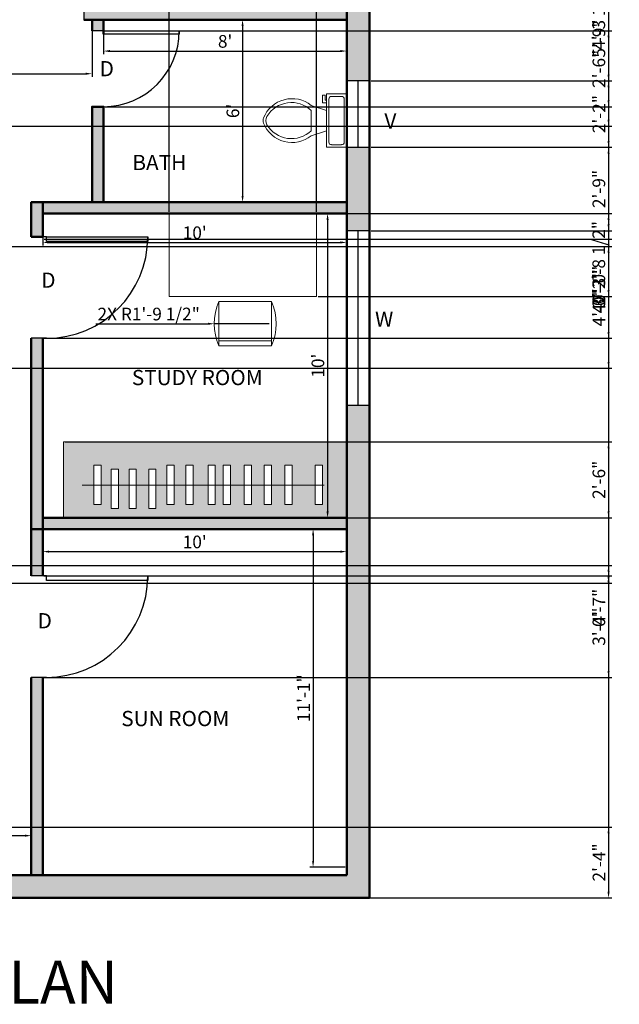
# Model space of a CAD drawing. Units: inches. Extents: x 2064 to 2999, y 1440 to 2089.
# Tile 6 of 7: x 2763 to 2999, y 1446 to 1835. Entities that reach past the tile are written whole.
import ezdxf

# ---------------------------------------------------------------- set-up
doc = ezdxf.new("R2010")
doc.units = ezdxf.units.IN
for name, color, linetype, lineweight in [('A-ANNO-DIMS', 2, 'Continuous', 18), ('A-ANNO-TEXT', 3, 'Continuous', 18), ('A-AREA-IDEN', 7, 'Continuous', 18), ('A-DOOR', 4, 'Continuous', 25), ('A-FLOR-FIXT', 9, 'Continuous', 18), ('A-FURN', 8, 'Continuous', 18), ('A-FURN-PATT', 252, 'Continuous', 13), ('A-GLAZ', 3, 'Continuous', 25), ('A-WALL', 7, 'Continuous', 50), ('A-WALL-PATT', 8, 'Continuous', 13)]:
    doc.layers.add(name, color=color, linetype=linetype, lineweight=lineweight)
doc.styles.get("Standard").update_dxf_attribs({"font": 'arial.ttf'})
doc.dimstyles.new('ISO-25', dxfattribs={"dimtxt": 5, "dimasz": 2.5, "dimexe": 1.25, "dimexo": 0.625, "dimtad": 1, "dimdec": 0, "dimlunit": 4, "dimtxsty": 'Standard', "dimcen": 2.5, "dimadec": 0, "dimazin": 0, "dimtfac": 1, "dimtdec": 0, "dimtmove": 0, "dimatfit": 3, "dimfxl": 1, "dimarcsym": 0})

# ---------------------------------------------------------------- blocks, each defined once
blk = doc.blocks.new('*U2')
for p, q in [((0, 0), (0, -6)), ((40, 0), (40, -6))]:
    blk.add_line(p, q)
blk.add_lwpolyline([(0, 0), (0, 40), (1.75, 40), (1.75, 0)], close=True)
blk.add_arc((0, 0), 40, 0, 90)
blk = doc.blocks.new('*U4')
for p, q in [((9.5, -6), (9.5, -2)), ((-10, -8.5), (-8, -8.5)), ((-10, -9.5), (-10, -8.5)), ((-7, -9.5), (-10, -9.5)), ((-8, -8.5), (-8, -8)), ((-7, -8), (-7, -9.5)), ((-4, -8), (-6, -14)), ((4, -8), (6, -14)), ((4, -14), (-4, -14))]:
    blk.add_line(p, q)
blk.add_lwpolyline([(10.5, -8), (10.5, 0), (-10.5, 0), (-10.5, -8)], close=True)
for points in [[(-9.5, -2), (-9.5, -6)], [(8.5, -1), (-8.5, -1)], [(-8.5, -7), (8.5, -7)]]:
    blk.add_lwpolyline(points)
for centre, radius, start, end in [((-8.62, -1.88), 0.884, 81.8699, 188.1301), ((8.62, -1.88), 0.884, 351.8699, 98.1301), ((-8.62, -6.12), 0.884, 171.8699, 278.1301), ((8.62, -6.12), 0.884, 261.8699, 8.1301), ((3.52, -21.58), 12.17, 141.4691, 247.9714), ((4.2, -21.82), 11.33, 136.3677, 238.9468), ((-3.52, -21.58), 12.17, 292.0284, 38.5307), ((-4.2, -21.82), 11.33, 301.053, 43.6321), ((0, -27.88), 4, 245.7318, 294.2682), ((0, -29), 4, 254.8605, 285.1395)]:
    blk.add_arc(centre, radius, start, end)
blk = doc.blocks.new('*D25')
at = {"layer": 'A-ANNO-DIMS', "color": 0, "lineweight": -2, "transparency": 16777216}
for p, q in [((2891.25, 1834.57), (2849.51, 1834.57)), ((2850.76, 1832.07), (2850.76, 1765.07)), ((2891.25, 1762.57), (2849.51, 1762.57))]:
    blk.add_line(p, q, dxfattribs=at)
at = {"layer": 'A-ANNO-DIMS', "color": 0, "transparency": 16777216}
for points in [[(2850.35, 1832.07), (2851.18, 1832.07), (2850.76, 1834.57)], [(2850.35, 1765.07), (2851.18, 1765.07), (2850.76, 1762.57)]]:
    blk.add_solid(points, dxfattribs=at)
at = {"layer": 'Defpoints', "color": 0, "transparency": 16777216}
for p in [(2891.87, 1834.57), (2850.76, 1762.57), (2891.87, 1762.57)]:
    blk.add_point(p, dxfattribs=at)
at = {"layer": 'A-ANNO-DIMS', "color": 0, "transparency": 16777216, "insert": (2847.58, 1798.57), "char_height": 5, "attachment_point": 5, "rotation": 90}
blk.add_mtext("6'", dxfattribs=at)
blk = doc.blocks.new('*D26')
at = {"layer": 'A-ANNO-DIMS', "color": 0, "lineweight": -2, "transparency": 16777216}
for p, q in [((2795.87, 1833.95), (2795.87, 1820.94)), ((2891.87, 1833.95), (2891.87, 1820.94)), ((2798.37, 1822.19), (2889.37, 1822.19))]:
    blk.add_line(p, q, dxfattribs=at)
at = {"layer": 'A-ANNO-DIMS', "color": 0, "transparency": 16777216}
for points in [[(2798.37, 1822.61), (2798.37, 1821.78), (2795.87, 1822.19)], [(2889.37, 1822.61), (2889.37, 1821.78), (2891.87, 1822.19)]]:
    blk.add_solid(points, dxfattribs=at)
at = {"layer": 'Defpoints', "color": 0, "transparency": 16777216}
for p in [(2795.87, 1834.57), (2891.87, 1834.57), (2891.87, 1822.19)]:
    blk.add_point(p, dxfattribs=at)
at = {"layer": 'A-ANNO-DIMS', "color": 0, "transparency": 16777216, "insert": (2843.87, 1825.37), "char_height": 5, "attachment_point": 5}
blk.add_mtext("8'", dxfattribs=at)
blk = doc.blocks.new('*D27')
at = {"layer": 'A-ANNO-DIMS', "color": 0, "lineweight": -2, "transparency": 16777216}
for p, q in [((2771.87, 1757.45), (2771.87, 1745.43)), ((2891.87, 1757.45), (2891.87, 1745.43)), ((2774.37, 1746.68), (2889.37, 1746.68))]:
    blk.add_line(p, q, dxfattribs=at)
at = {"layer": 'A-ANNO-DIMS', "color": 0, "transparency": 16777216}
for points in [[(2774.37, 1747.1), (2774.37, 1746.27), (2771.87, 1746.68)], [(2889.37, 1747.1), (2889.37, 1746.27), (2891.87, 1746.68)]]:
    blk.add_solid(points, dxfattribs=at)
at = {"layer": 'Defpoints', "color": 0, "transparency": 16777216}
for p in [(2771.87, 1758.07), (2891.87, 1758.07), (2891.87, 1746.68)]:
    blk.add_point(p, dxfattribs=at)
at = {"layer": 'A-ANNO-DIMS', "color": 0, "transparency": 16777216, "insert": (2831.87, 1749.86), "char_height": 5, "attachment_point": 5}
blk.add_mtext("10'", dxfattribs=at)
blk = doc.blocks.new('*D28')
at = {"layer": 'A-ANNO-DIMS', "color": 0, "lineweight": -2, "transparency": 16777216}
for p, q in [((2891.25, 1758.07), (2883.07, 1758.07)), ((2884.32, 1755.57), (2884.32, 1640.57)), ((2891.25, 1638.07), (2883.07, 1638.07))]:
    blk.add_line(p, q, dxfattribs=at)
at = {"layer": 'A-ANNO-DIMS', "color": 0, "transparency": 16777216}
for points in [[(2883.9, 1755.57), (2884.73, 1755.57), (2884.32, 1758.07)], [(2883.9, 1640.57), (2884.73, 1640.57), (2884.32, 1638.07)]]:
    blk.add_solid(points, dxfattribs=at)
at = {"layer": 'Defpoints', "color": 0, "transparency": 16777216}
for p in [(2891.87, 1758.07), (2884.32, 1638.07), (2891.87, 1638.07)]:
    blk.add_point(p, dxfattribs=at)
at = {"layer": 'A-ANNO-DIMS', "color": 0, "transparency": 16777216, "insert": (2881.14, 1698.07), "char_height": 5, "attachment_point": 5, "rotation": 90}
blk.add_mtext("10'", dxfattribs=at)
blk = doc.blocks.new('*D29')
at = {"layer": 'A-ANNO-DIMS', "color": 0, "lineweight": -2, "transparency": 16777216}
for p, q in [((2771.87, 1632.95), (2771.87, 1623.44)), ((2891.87, 1632.95), (2891.87, 1623.44)), ((2774.37, 1624.69), (2889.37, 1624.69))]:
    blk.add_line(p, q, dxfattribs=at)
at = {"layer": 'A-ANNO-DIMS', "color": 0, "transparency": 16777216}
for points in [[(2774.37, 1625.1), (2774.37, 1624.27), (2771.87, 1624.69)], [(2889.37, 1625.1), (2889.37, 1624.27), (2891.87, 1624.69)]]:
    blk.add_solid(points, dxfattribs=at)
at = {"layer": 'Defpoints', "color": 0, "transparency": 16777216}
for p in [(2771.87, 1633.57), (2891.87, 1633.57), (2891.87, 1624.69)]:
    blk.add_point(p, dxfattribs=at)
at = {"layer": 'A-ANNO-DIMS', "color": 0, "transparency": 16777216, "insert": (2831.87, 1627.86), "char_height": 5, "attachment_point": 5}
blk.add_mtext("10'", dxfattribs=at)
blk = doc.blocks.new('*D30')
at = {"layer": 'A-ANNO-DIMS', "color": 0, "lineweight": -2, "transparency": 16777216}
for p, q in [((2891.25, 1633.57), (2877.35, 1633.57)), ((2878.6, 1631.07), (2878.6, 1502.68)), ((2891.25, 1500.18), (2877.35, 1500.18))]:
    blk.add_line(p, q, dxfattribs=at)
at = {"layer": 'A-ANNO-DIMS', "color": 0, "transparency": 16777216}
for points in [[(2878.19, 1631.07), (2879.02, 1631.07), (2878.6, 1633.57)], [(2878.19, 1502.68), (2879.02, 1502.68), (2878.6, 1500.18)]]:
    blk.add_solid(points, dxfattribs=at)
at = {"layer": 'Defpoints', "color": 0, "transparency": 16777216}
for p in [(2891.87, 1633.57), (2878.6, 1500.18), (2891.87, 1500.18)]:
    blk.add_point(p, dxfattribs=at)
at = {"layer": 'A-ANNO-DIMS', "color": 0, "transparency": 16777216, "insert": (2875.47, 1566.88), "char_height": 5, "attachment_point": 5, "rotation": 90}
blk.add_mtext('11\'-1"', dxfattribs=at)
blk = doc.blocks.new('*D31')
at = {"layer": 'A-ANNO-DIMS', "color": 0, "lineweight": -2, "transparency": 16777216}
for p, q in [((2549.87, 1497.7), (2549.87, 1513.87)), ((2552.37, 1512.62), (2764.87, 1512.62)), ((2767.37, 1497.7), (2767.37, 1513.87))]:
    blk.add_line(p, q, dxfattribs=at)
at = {"layer": 'A-ANNO-DIMS', "color": 0, "transparency": 16777216}
for points in [[(2552.37, 1513.04), (2552.37, 1512.2), (2549.87, 1512.62)], [(2764.87, 1513.04), (2764.87, 1512.2), (2767.37, 1512.62)]]:
    blk.add_solid(points, dxfattribs=at)
at = {"layer": 'Defpoints', "color": 0, "transparency": 16777216}
for p in [(2767.37, 1512.62), (2549.87, 1497.07), (2767.37, 1497.07)]:
    blk.add_point(p, dxfattribs=at)
at = {"layer": 'A-ANNO-DIMS', "color": 0, "transparency": 16777216, "insert": (2658.62, 1515.8), "char_height": 5, "attachment_point": 5}
blk.add_mtext('18\'-2"', dxfattribs=at)
blk = doc.blocks.new('*D33')
at = {"layer": 'A-ANNO-DIMS', "color": 0, "lineweight": -2, "transparency": 16777216}
for p, q in [((2616.69, 1833.95), (2616.69, 1812)), ((2791.37, 1833.95), (2791.37, 1812)), ((2619.19, 1813.25), (2788.87, 1813.25))]:
    blk.add_line(p, q, dxfattribs=at)
at = {"layer": 'A-ANNO-DIMS', "color": 0, "transparency": 16777216}
for points in [[(2619.19, 1813.67), (2619.19, 1812.84), (2616.69, 1813.25)], [(2788.87, 1813.67), (2788.87, 1812.84), (2791.37, 1813.25)]]:
    blk.add_solid(points, dxfattribs=at)
at = {"layer": 'Defpoints', "color": 0, "transparency": 16777216}
for p in [(2616.69, 1834.57), (2791.37, 1834.57), (2791.37, 1813.25)]:
    blk.add_point(p, dxfattribs=at)
at = {"layer": 'A-ANNO-DIMS', "color": 0, "transparency": 16777216, "insert": (2704.03, 1816.39), "char_height": 5, "attachment_point": 5}
blk.add_mtext('14\'-7"', dxfattribs=at)
blk = doc.blocks.new('BOOK')
for p, q in [((0, 3.13), (0, 15.5)), ((0, 15.5), (0, 0)), ((2.86, 15.5), (0, 15.5)), ((2.86, 0), (2.86, 15.5)), ((0, 0), (2.86, 0))]:
    blk.add_line(p, q)
blk = doc.blocks.new('WIN-69')
blk.add_line((4.5, 0), (4.5, 68.8))
blk.add_lwpolyline([(0, 0), (9, 0), (9, 68.8), (0, 68.8)], close=True)
blk = doc.blocks.new('*D83')
at = {"layer": 'A-ANNO-DIMS', "color": 0, "lineweight": -2, "transparency": 16777216}
for p, q in [((2901.5, 1968.07), (2996.47, 1968.07)), ((2995.22, 1965.57), (2995.22, 1490.57)), ((2901.5, 1488.07), (2996.47, 1488.07))]:
    blk.add_line(p, q, dxfattribs=at)
at = {"layer": 'A-ANNO-DIMS', "color": 0, "transparency": 16777216}
for points in [[(2994.81, 1965.57), (2995.64, 1965.57), (2995.22, 1968.07)], [(2994.81, 1490.57), (2995.64, 1490.57), (2995.22, 1488.07)]]:
    blk.add_solid(points, dxfattribs=at)
at = {"layer": 'Defpoints', "color": 0, "transparency": 16777216}
for p in [(2900.87, 1968.07), (2900.87, 1488.07), (2995.22, 1488.07)]:
    blk.add_point(p, dxfattribs=at)
at = {"layer": 'A-ANNO-DIMS', "color": 0, "transparency": 16777216, "insert": (2992.05, 1728.07), "char_height": 5, "attachment_point": 5, "rotation": 90}
blk.add_mtext('40\'-0"', dxfattribs=at)
blk = doc.blocks.new('*D88')
at = {"layer": 'A-ANNO-DIMS', "color": 0, "lineweight": -2, "transparency": 16777216}
for p, q in [((2901.5, 1861.72), (2996.47, 1861.72)), ((2995.22, 1859.22), (2995.22, 1812.91)), ((2901.5, 1810.41), (2996.47, 1810.41))]:
    blk.add_line(p, q, dxfattribs=at)
at = {"layer": 'A-ANNO-DIMS', "color": 0, "transparency": 16777216}
for points in [[(2994.81, 1859.22), (2995.64, 1859.22), (2995.22, 1861.72)], [(2994.81, 1812.91), (2995.64, 1812.91), (2995.22, 1810.41)]]:
    blk.add_solid(points, dxfattribs=at)
at = {"layer": 'Defpoints', "color": 0, "transparency": 16777216}
for p in [(2900.87, 1861.72), (2900.87, 1810.41), (2995.22, 1810.41)]:
    blk.add_point(p, dxfattribs=at)
at = {"layer": 'A-ANNO-DIMS', "color": 0, "transparency": 16777216, "insert": (2992.01, 1836.07), "char_height": 5, "attachment_point": 5, "rotation": 90}
blk.add_mtext('4\'-3 1/2"', dxfattribs=at)
blk = doc.blocks.new('*D89')
at = {"layer": 'A-ANNO-DIMS', "color": 0, "lineweight": -2, "transparency": 16777216}
for p, q in [((2901.5, 1810.41), (2996.47, 1810.41)), ((2995.22, 1807.91), (2995.22, 1786.76)), ((2901.5, 1784.26), (2996.47, 1784.26))]:
    blk.add_line(p, q, dxfattribs=at)
at = {"layer": 'A-ANNO-DIMS', "color": 0, "transparency": 16777216}
for points in [[(2994.81, 1807.91), (2995.64, 1807.91), (2995.22, 1810.41)], [(2994.81, 1786.76), (2995.64, 1786.76), (2995.22, 1784.26)]]:
    blk.add_solid(points, dxfattribs=at)
at = {"layer": 'Defpoints', "color": 0, "transparency": 16777216}
for p in [(2900.87, 1810.41), (2900.87, 1784.26), (2995.22, 1784.26)]:
    blk.add_point(p, dxfattribs=at)
at = {"layer": 'A-ANNO-DIMS', "color": 0, "transparency": 16777216, "insert": (2992.09, 1797.33), "char_height": 5, "attachment_point": 5, "rotation": 90}
blk.add_mtext('2\'-2"', dxfattribs=at)
blk = doc.blocks.new('*D90')
at = {"layer": 'A-ANNO-DIMS', "color": 0, "lineweight": -2, "transparency": 16777216}
for p, q in [((2901.5, 1784.26), (2996.47, 1784.26)), ((2995.22, 1781.76), (2995.22, 1753.81)), ((2901.5, 1751.31), (2996.47, 1751.31))]:
    blk.add_line(p, q, dxfattribs=at)
at = {"layer": 'A-ANNO-DIMS', "color": 0, "transparency": 16777216}
for points in [[(2994.81, 1781.76), (2995.64, 1781.76), (2995.22, 1784.26)], [(2994.81, 1753.81), (2995.64, 1753.81), (2995.22, 1751.31)]]:
    blk.add_solid(points, dxfattribs=at)
at = {"layer": 'Defpoints', "color": 0, "transparency": 16777216}
for p in [(2900.87, 1784.26), (2900.87, 1751.31), (2995.22, 1751.31)]:
    blk.add_point(p, dxfattribs=at)
at = {"layer": 'A-ANNO-DIMS', "color": 0, "transparency": 16777216, "insert": (2992.05, 1767.78), "char_height": 5, "attachment_point": 5, "rotation": 90}
blk.add_mtext('2\'-9"', dxfattribs=at)
blk = doc.blocks.new('*D92')
at = {"layer": 'A-ANNO-DIMS', "color": 0, "lineweight": -2, "transparency": 16777216}
for p, q in [((2541.5, 1861.72), (2996.47, 1861.72)), ((2995.22, 1859.22), (2995.22, 1795.07)), ((2541.5, 1792.57), (2996.47, 1792.57))]:
    blk.add_line(p, q, dxfattribs=at)
at = {"layer": 'A-ANNO-DIMS', "color": 0, "transparency": 16777216}
for points in [[(2994.81, 1859.22), (2995.64, 1859.22), (2995.22, 1861.72)], [(2994.81, 1795.07), (2995.64, 1795.07), (2995.22, 1792.57)]]:
    blk.add_solid(points, dxfattribs=at)
at = {"layer": 'Defpoints', "color": 0, "transparency": 16777216}
for p in [(2540.87, 1861.72), (2540.87, 1792.57), (2995.22, 1792.57)]:
    blk.add_point(p, dxfattribs=at)
at = {"layer": 'A-ANNO-DIMS', "color": 0, "transparency": 16777216, "insert": (2992.05, 1827.15), "char_height": 5, "attachment_point": 5, "rotation": 90}
blk.add_mtext('5\'-9"', dxfattribs=at)
blk = doc.blocks.new('*D93')
at = {"layer": 'A-ANNO-DIMS', "color": 0, "lineweight": -2, "transparency": 16777216}
for p, q in [((2541.5, 1745.09), (2996.47, 1745.09)), ((2995.22, 1742.59), (2995.22, 1699.57)), ((2541.5, 1697.07), (2996.47, 1697.07))]:
    blk.add_line(p, q, dxfattribs=at)
at = {"layer": 'A-ANNO-DIMS', "color": 0, "transparency": 16777216}
for points in [[(2994.81, 1742.59), (2995.64, 1742.59), (2995.22, 1745.09)], [(2994.81, 1699.57), (2995.64, 1699.57), (2995.22, 1697.07)]]:
    blk.add_solid(points, dxfattribs=at)
at = {"layer": 'Defpoints', "color": 0, "transparency": 16777216}
for p in [(2540.87, 1745.09), (2540.87, 1697.07), (2995.22, 1697.07)]:
    blk.add_point(p, dxfattribs=at)
at = {"layer": 'A-ANNO-DIMS', "color": 0, "transparency": 16777216, "insert": (2992.05, 1721.08), "char_height": 5, "attachment_point": 5, "rotation": 90}
blk.add_mtext('4\'-0"', dxfattribs=at)
blk = doc.blocks.new('*D94')
at = {"layer": 'A-ANNO-DIMS', "color": 0, "lineweight": -2, "transparency": 16777216}
for p, q in [((2541.5, 1619.25), (2996.47, 1619.25)), ((2995.22, 1616.75), (2995.22, 1614.76)), ((2541.5, 1612.26), (2996.47, 1612.26)), ((2995.22, 1612.26), (2995.22, 1595.22))]:
    blk.add_line(p, q, dxfattribs=at)
at = {"layer": 'A-ANNO-DIMS', "color": 0, "transparency": 16777216}
for points in [[(2994.81, 1616.75), (2995.64, 1616.75), (2995.22, 1619.25)], [(2994.81, 1614.76), (2995.64, 1614.76), (2995.22, 1612.26)]]:
    blk.add_solid(points, dxfattribs=at)
at = {"layer": 'Defpoints', "color": 0, "transparency": 16777216}
for p in [(2540.87, 1619.25), (2540.87, 1612.26), (2995.22, 1612.26)]:
    blk.add_point(p, dxfattribs=at)
at = {"layer": 'A-ANNO-DIMS', "color": 0, "transparency": 16777216, "insert": (2992.05, 1602.49), "char_height": 5, "attachment_point": 5, "rotation": 90}
blk.add_mtext('0\'-7"', dxfattribs=at)
blk = doc.blocks.new('*D95')
at = {"layer": 'A-ANNO-DIMS', "color": 0, "lineweight": -2, "transparency": 16777216}
for p, q in [((2541.5, 1516.02), (2996.47, 1516.02)), ((2995.22, 1513.52), (2995.22, 1490.57)), ((2541.5, 1488.07), (2996.47, 1488.07))]:
    blk.add_line(p, q, dxfattribs=at)
at = {"layer": 'A-ANNO-DIMS', "color": 0, "transparency": 16777216}
for points in [[(2994.81, 1513.52), (2995.64, 1513.52), (2995.22, 1516.02)], [(2994.81, 1490.57), (2995.64, 1490.57), (2995.22, 1488.07)]]:
    blk.add_solid(points, dxfattribs=at)
at = {"layer": 'Defpoints', "color": 0, "transparency": 16777216}
for p in [(2540.87, 1516.02), (2540.87, 1488.07), (2995.22, 1488.07)]:
    blk.add_point(p, dxfattribs=at)
at = {"layer": 'A-ANNO-DIMS', "color": 0, "transparency": 16777216, "insert": (2992.09, 1502.05), "char_height": 5, "attachment_point": 5, "rotation": 90}
blk.add_mtext('2\'-4"', dxfattribs=at)
blk = doc.blocks.new('*D104')
at = {"layer": 'A-ANNO-DIMS', "color": 0, "lineweight": -2, "transparency": 16777216}
for p, q in [((2821.8, 1758.7), (2821.8, 2012.67)), ((2879.97, 1758.7), (2879.97, 2012.67)), ((2824.3, 2011.42), (2877.47, 2011.42))]:
    blk.add_line(p, q, dxfattribs=at)
at = {"layer": 'A-ANNO-DIMS', "color": 0, "transparency": 16777216}
for points in [[(2824.3, 2011.84), (2824.3, 2011), (2821.8, 2011.42)], [(2877.47, 2011.84), (2877.47, 2011), (2879.97, 2011.42)]]:
    blk.add_solid(points, dxfattribs=at)
at = {"layer": 'Defpoints', "color": 0, "transparency": 16777216}
for p in [(2879.97, 2011.42), (2821.8, 1758.07), (2879.97, 1758.07)]:
    blk.add_point(p, dxfattribs=at)
at = {"layer": 'A-ANNO-DIMS', "color": 0, "transparency": 16777216, "insert": (2850.89, 2014.6), "char_height": 5, "attachment_point": 5}
blk.add_mtext('4\'-10"', dxfattribs=at)
blk = doc.blocks.new('*D105')
at = {"layer": 'A-ANNO-DIMS', "color": 0, "lineweight": -2, "transparency": 16777216}
for p, q in [((2880.6, 1758.07), (2996.47, 1758.07)), ((2995.22, 1755.57), (2995.22, 1727.87)), ((2880.6, 1725.37), (2996.47, 1725.37))]:
    blk.add_line(p, q, dxfattribs=at)
at = {"layer": 'A-ANNO-DIMS', "color": 0, "transparency": 16777216}
for points in [[(2994.81, 1755.57), (2995.64, 1755.57), (2995.22, 1758.07)], [(2994.81, 1727.87), (2995.64, 1727.87), (2995.22, 1725.37)]]:
    blk.add_solid(points, dxfattribs=at)
at = {"layer": 'Defpoints', "color": 0, "transparency": 16777216}
for p in [(2879.97, 1758.07), (2879.97, 1725.37), (2995.22, 1725.37)]:
    blk.add_point(p, dxfattribs=at)
at = {"layer": 'A-ANNO-DIMS', "color": 0, "transparency": 16777216, "insert": (2992.01, 1741.72), "char_height": 5, "attachment_point": 5, "rotation": 90}
blk.add_mtext('2\'-8 1/2"', dxfattribs=at)
blk = doc.blocks.new('*D106')
at = {"layer": 'A-ANNO-DIMS', "color": 0, "lineweight": -2, "transparency": 16777216}
for p, q in [((2780.75, 1667.99), (2996.47, 1667.99)), ((2995.22, 1665.49), (2995.22, 1640.57)), ((2780.75, 1638.07), (2996.47, 1638.07))]:
    blk.add_line(p, q, dxfattribs=at)
at = {"layer": 'A-ANNO-DIMS', "color": 0, "transparency": 16777216}
for points in [[(2994.81, 1665.49), (2995.64, 1665.49), (2995.22, 1667.99)], [(2994.81, 1640.57), (2995.64, 1640.57), (2995.22, 1638.07)]]:
    blk.add_solid(points, dxfattribs=at)
at = {"layer": 'Defpoints', "color": 0, "transparency": 16777216}
for p in [(2780.13, 1667.99), (2780.13, 1638.07), (2995.22, 1638.07)]:
    blk.add_point(p, dxfattribs=at)
at = {"layer": 'A-ANNO-DIMS', "color": 0, "transparency": 16777216, "insert": (2992.05, 1653.03), "char_height": 5, "attachment_point": 5, "rotation": 90}
blk.add_mtext('2\'-6"', dxfattribs=at)
blk = doc.blocks.new('*D117')
at = {"layer": 'A-ANNO-DIMS', "color": 0, "lineweight": -2, "transparency": 16777216}
for p, q in [((2796.48, 1830.13), (2996.47, 1830.13)), ((2995.22, 1827.63), (2995.22, 1802.73)), ((2796.48, 1800.23), (2996.47, 1800.23))]:
    blk.add_line(p, q, dxfattribs=at)
at = {"layer": 'A-ANNO-DIMS', "color": 0, "transparency": 16777216}
for points in [[(2994.81, 1827.63), (2995.64, 1827.63), (2995.22, 1830.13)], [(2994.81, 1802.73), (2995.64, 1802.73), (2995.22, 1800.23)]]:
    blk.add_solid(points, dxfattribs=at)
at = {"layer": 'Defpoints', "color": 0, "transparency": 16777216}
for p in [(2795.86, 1830.13), (2795.86, 1800.23), (2995.22, 1800.23)]:
    blk.add_point(p, dxfattribs=at)
at = {"layer": 'A-ANNO-DIMS', "color": 0, "transparency": 16777216, "insert": (2992.05, 1815.18), "char_height": 5, "attachment_point": 5, "rotation": 90}
blk.add_mtext('2\'-6"', dxfattribs=at)
blk = doc.blocks.new('*D118')
at = {"layer": 'A-ANNO-DIMS', "color": 0, "lineweight": -2, "transparency": 16777216}
for p, q in [((2772.48, 1747.98), (2996.47, 1747.98)), ((2995.22, 1745.48), (2995.22, 1711.35)), ((2772.25, 1708.85), (2996.47, 1708.85))]:
    blk.add_line(p, q, dxfattribs=at)
at = {"layer": 'A-ANNO-DIMS', "color": 0, "transparency": 16777216}
for points in [[(2994.81, 1745.48), (2995.64, 1745.48), (2995.22, 1747.98)], [(2994.81, 1711.35), (2995.64, 1711.35), (2995.22, 1708.85)]]:
    blk.add_solid(points, dxfattribs=at)
at = {"layer": 'Defpoints', "color": 0, "transparency": 16777216}
for p in [(2771.86, 1747.98), (2771.62, 1708.85), (2995.22, 1708.85)]:
    blk.add_point(p, dxfattribs=at)
at = {"layer": 'A-ANNO-DIMS', "color": 0, "transparency": 16777216, "insert": (2992.05, 1728.42), "char_height": 5, "attachment_point": 5, "rotation": 90}
blk.add_mtext('3\'-3"', dxfattribs=at)
blk = doc.blocks.new('*D119')
at = {"layer": 'A-ANNO-DIMS', "color": 0, "lineweight": -2, "transparency": 16777216}
for p, q in [((2772.25, 1615.08), (2996.47, 1615.08)), ((2995.22, 1612.58), (2995.22, 1577.58)), ((2772.25, 1575.08), (2996.47, 1575.08))]:
    blk.add_line(p, q, dxfattribs=at)
at = {"layer": 'A-ANNO-DIMS', "color": 0, "transparency": 16777216}
for points in [[(2994.81, 1612.58), (2995.64, 1612.58), (2995.22, 1615.08)], [(2994.81, 1577.58), (2995.64, 1577.58), (2995.22, 1575.08)]]:
    blk.add_solid(points, dxfattribs=at)
at = {"layer": 'Defpoints', "color": 0, "transparency": 16777216}
for p in [(2771.62, 1615.08), (2771.62, 1575.08), (2995.22, 1575.08)]:
    blk.add_point(p, dxfattribs=at)
at = {"layer": 'A-ANNO-DIMS', "color": 0, "transparency": 16777216, "insert": (2992.05, 1595.08), "char_height": 5, "attachment_point": 5, "rotation": 90}
blk.add_mtext('3\'-4"', dxfattribs=at)
blk = doc.blocks.new('*D120')
at = {"layer": 'A-ANNO-DIMS', "color": 0, "lineweight": -2, "transparency": 16777216}
for p, q in [((2792.81, 1714.55), (2837.11, 1714.6)), ((2861.25, 1714.62), (2839.61, 1714.6))]:
    blk.add_line(p, q, dxfattribs=at)
at = {"layer": 'A-ANNO-DIMS', "color": 0, "transparency": 16777216}
blk.add_solid([(2837.11, 1715.01), (2837.11, 1714.18), (2839.61, 1714.6)], dxfattribs=at)
at = {"layer": 'Defpoints', "color": 0, "transparency": 16777216}
for p in [(2839.61, 1714.6), (2861.25, 1714.62)]:
    blk.add_point(p, dxfattribs=at)
at = {"layer": 'A-ANNO-DIMS', "color": 0, "transparency": 16777216, "insert": (2813.71, 1717.78), "char_height": 5, "attachment_point": 5, "rotation": 0.0598}
blk.add_mtext('2X R1\'-9 1/2"', dxfattribs=at)

msp = doc.modelspace()

# ---------------------------------------------------------------- hatches: boundary and pattern name
at = {"layer": 'A-FURN-PATT'}
h = msp.add_hatch(color=256, dxfattribs=at)
h.dxf.hatch_style = 1
h.paths.add_polyline_path([(2211.98, 1959.07), (2126.82, 1959.07), (2126.82, 1938.57), (2211.98, 1938.57)])
h.paths.add_polyline_path([(2669.87, 1959.07), (2646.96, 1959.07), (2646.96, 1892.49), (2669.87, 1892.49)])
h.paths.add_polyline_path([(2468.82, 1668.53), (2348.82, 1668.53), (2348.82, 1638.07), (2468.82, 1638.07)])
h.paths.add_polyline_path([(2891.87, 1667.99), (2780.13, 1667.99), (2780.13, 1638.07), (2891.87, 1638.07)])
h.paths.add_polyline_path([(2854.27, 1658.75), (2854.27, 1650.97), (2859.31, 1650.97), (2859.31, 1658.75), (2862.16, 1658.75), (2862.16, 1650.97), (2867.47, 1650.97), (2867.47, 1658.75), (2870.33, 1658.75), (2870.33, 1650.97), (2879.45, 1650.97), (2879.45, 1658.75), (2882.31, 1658.75), (2882.31, 1643.24), (2879.45, 1643.24), (2879.45, 1650.97), (2870.33, 1650.97), (2870.33, 1643.24), (2867.47, 1643.24), (2867.47, 1650.97), (2862.16, 1650.97), (2862.16, 1643.24), (2859.31, 1643.24), (2859.31, 1650.97), (2854.27, 1650.97), (2854.27, 1643.24), (2851.41, 1643.24), (2851.41, 1650.97), (2845.97, 1650.97), (2845.97, 1643.24), (2843.11, 1643.24), (2843.11, 1650.97), (2839.98, 1650.97), (2839.98, 1643.24), (2837.12, 1643.24), (2837.12, 1650.97), (2831.27, 1650.97), (2831.27, 1643.24), (2828.41, 1643.24), (2828.41, 1650.97), (2823.78, 1650.97), (2823.78, 1643.24), (2820.92, 1643.24), (2820.92, 1650.97), (2816.56, 1650.97), (2816.56, 1641.66), (2813.71, 1641.66), (2813.71, 1650.97), (2808.81, 1650.97), (2808.81, 1641.66), (2805.95, 1641.66), (2805.95, 1650.97), (2801.73, 1650.97), (2801.73, 1641.66), (2798.87, 1641.66), (2798.87, 1650.97), (2794.92, 1650.97), (2794.92, 1643.24), (2792.06, 1643.24), (2792.06, 1658.75), (2794.92, 1658.75), (2794.92, 1650.97), (2798.87, 1650.97), (2798.87, 1657.16), (2801.73, 1657.16), (2801.73, 1650.97), (2805.95, 1650.97), (2805.95, 1657.16), (2808.81, 1657.16), (2808.81, 1650.97), (2813.71, 1650.97), (2813.71, 1657.16), (2816.56, 1657.16), (2816.56, 1650.97), (2820.92, 1650.97), (2820.92, 1658.75), (2823.78, 1658.75), (2823.78, 1650.97), (2828.41, 1650.97), (2828.41, 1658.75), (2831.27, 1658.75), (2831.27, 1650.97), (2837.12, 1650.97), (2837.12, 1658.75), (2839.98, 1658.75), (2839.98, 1650.97), (2843.11, 1650.97), (2843.11, 1658.75), (2845.97, 1658.75), (2845.97, 1650.97), (2851.41, 1650.97), (2851.41, 1658.75)], flags=16)
h.paths.add_polyline_path([(2665.84, 1899.31), (2665.84, 1951.8), (2653.45, 1951.8), (2653.45, 1899.31)], flags=24)
h.paths.add_polyline_path([(2565.91, 1921.55), (2649.69, 1921.55), (2649.69, 1933.95), (2565.91, 1933.95)], flags=9)
h.paths.add_polyline_path([(2402.8, 1649), (2414.4, 1649), (2414.4, 1659.3), (2402.8, 1659.3)], flags=24)
at = {"layer": 'A-WALL-PATT'}
h = msp.add_hatch(color=256, dxfattribs=at)
h.dxf.hatch_style = 1
h.paths.add_polyline_path([(2574.52, 1968.07), (2540.87, 1968.07), (2540.87, 1930.52), (2549.87, 1930.52), (2549.87, 1959.07), (2574.52, 1959.07)])
h.paths.add_polyline_path([(2687.51, 1968.07), (2643.06, 1968.07), (2643.06, 1959.07), (2669.87, 1959.07), (2687.51, 1959.07)])
h.paths.add_polyline_path([(2900.87, 1968.07), (2728.11, 1968.07), (2728.11, 1959.07), (2740.37, 1959.07), (2891.87, 1959.07), (2891.87, 1930.52), (2900.87, 1930.52)])
h.paths.add_polyline_path([(2744.87, 1959.07), (2740.37, 1959.07), (2740.37, 1839.07), (2674.37, 1839.07), (2674.37, 1959.07), (2669.87, 1959.07), (2669.87, 1892.49), (2669.87, 1839.07), (2665.15, 1839.07), (2665.15, 1834.57), (2674.37, 1834.57), (2744.87, 1834.57), (2748.11, 1834.57), (2748.11, 1839.07), (2744.87, 1839.07)])
h.paths.add_polyline_path([(2549.87, 1834.57), (2549.87, 1861.72), (2540.87, 1861.72), (2540.87, 1792.57), (2549.87, 1792.57)])
h.paths.add_polyline_path([(2625.15, 1839.07), (2549.87, 1839.07), (2549.87, 1834.57), (2625.15, 1834.57)])
h.paths.add_polyline_path([(2900.87, 1861.72), (2891.87, 1861.72), (2891.87, 1810.41), (2900.87, 1810.41)])
h.paths.add_polyline_path([(2891.87, 1839.07), (2788.11, 1839.07), (2788.11, 1834.57), (2891.87, 1834.57)])
h.paths.add_polyline_path([(2549.87, 1745.09), (2540.87, 1745.09), (2540.87, 1697.07), (2549.87, 1697.07)])
h.paths.add_polyline_path([(2549.87, 1619.25), (2540.87, 1619.25), (2540.87, 1612.26), (2549.87, 1612.26)], flags=17)
h.paths.add_polyline_path([(2549.87, 1516.02), (2540.87, 1516.02), (2540.87, 1488.07), (2900.87, 1488.07), (2900.87, 1682.51), (2891.87, 1682.51), (2891.87, 1497.07), (2549.87, 1497.07)])
h.paths.add_polyline_path([(2771.87, 1575.08), (2767.37, 1575.08), (2767.37, 1497.07), (2771.87, 1497.07)], flags=17)
h.paths.add_polyline_path([(2771.87, 1708.85), (2767.37, 1708.85), (2767.37, 1633.57), (2771.87, 1633.57), (2771.87, 1638.07)])
h.paths.add_polyline_path([(2891.87, 1638.07), (2780.13, 1638.07), (2771.87, 1638.07), (2771.87, 1633.57), (2891.87, 1633.57)], flags=17)
h.paths.add_polyline_path([(2771.87, 1633.57), (2767.37, 1633.57), (2767.37, 1615.08), (2771.87, 1615.08)], flags=17)
h.paths.add_polyline_path([(2900.87, 1784.26), (2891.87, 1784.26), (2891.87, 1751.31), (2900.87, 1751.31)])
h.paths.add_polyline_path([(2795.87, 1834.57), (2791.37, 1834.57), (2791.37, 1830.13), (2795.87, 1830.13)])
h.paths.add_polyline_path([(2805.14, 1771.92), (2830.56, 1771.92), (2830.56, 1784.32), (2805.14, 1784.32)], flags=9)
h.paths.add_polyline_path([(2805.18, 1686.98), (2865.14, 1686.98), (2865.14, 1699.38), (2805.18, 1699.38)], flags=9)
h.paths.add_polyline_path([(2801, 1552.43), (2850.22, 1552.43), (2850.22, 1564.83), (2801, 1564.83)], flags=25)
h.paths.add_polyline_path([(2645.3, 1586.75), (2705.73, 1586.75), (2705.73, 1599.14), (2645.3, 1599.14)], flags=25)
h.paths.add_polyline_path([(2670.49, 1736.4), (2713.67, 1736.4), (2713.67, 1748.79), (2670.49, 1748.79)], flags=9)
h.paths.add_polyline_path([(2795.9, 1895.95), (2857.73, 1895.95), (2857.73, 1908.34), (2795.9, 1908.34)], flags=9)
h.paths.add_polyline_path([(2565.91, 1921.55), (2649.69, 1921.55), (2649.69, 1933.95), (2565.91, 1933.95)], flags=9)
h = msp.add_hatch(color=256, dxfattribs=at)
h.dxf.hatch_style = 1
h.paths.add_polyline_path([(2891.87, 1762.57), (2771.87, 1762.57), (2771.87, 1758.07), (2891.87, 1758.07)])
h.paths.add_polyline_path([(2795.87, 1800.23), (2791.37, 1800.23), (2791.37, 1762.57), (2795.87, 1762.57)])
h.paths.add_polyline_path([(2771.87, 1762.57), (2767.37, 1762.57), (2767.37, 1748.85), (2771.87, 1748.85)])

# ---------------------------------------------------------------- linework, layer by layer
at = {"layer": 'A-FURN'}
for p, q in [((2841.45, 1707.9), (2862.2, 1707.9)), ((2787.43, 1650.97), (2883.01, 1650.97))]:
    msp.add_line(p, q, dxfattribs=at)
for points in [[(2821.8, 1758.07), (2879.97, 1758.07), (2879.97, 1725.37), (2821.8, 1725.37)], [(2841.45, 1723.35), (2862.2, 1723.35), (2862.2, 1705.89), (2841.45, 1705.89)], [(2780.13, 1638.07), (2891.87, 1638.07), (2891.87, 1667.99), (2780.13, 1667.99)]]:
    msp.add_lwpolyline(points, close=True, dxfattribs=at)
for centre, start, end in [((2861.25, 1714.62), 156.2089, 203.7911), ((2842.39, 1714.62), 336.2089, 23.7911)]:
    msp.add_arc(centre, 21.64, start, end, dxfattribs=at)
at = {"layer": 'A-GLAZ'}
msp.add_line((2896.37, 1784.26), (2896.37, 1810.41), dxfattribs=at)
msp.add_lwpolyline([(2891.87, 1784.26), (2900.87, 1784.26), (2900.87, 1810.41), (2891.87, 1810.41)], close=True, dxfattribs=at)
at = {"layer": 'A-WALL'}
for p, q in [((2900.87, 1968.07), (2900.87, 1488.07)), ((2891.87, 1959.07), (2891.87, 1497.07)), ((2788.11, 1834.57), (2891.87, 1834.57)), ((2791.37, 1834.57), (2791.37, 1830.13)), ((2891.87, 1834.57), (2795.87, 1834.57)), ((2795.87, 1834.57), (2795.87, 1828.82)), ((2891.87, 1834.57), (2891.87, 1738.57)), ((2791.37, 1800.23), (2791.37, 1762.57)), ((2795.87, 1800.23), (2795.87, 1762.57)), ((2767.37, 1762.57), (2767.37, 1748.85)), ((2791.37, 1762.57), (2767.37, 1762.57)), ((2795.87, 1762.57), (2891.87, 1762.57)), ((2891.87, 1762.57), (2795.87, 1762.57)), ((2791.37, 1758.07), (2771.87, 1758.07)), ((2771.87, 1758.07), (2771.87, 1748.85)), ((2791.37, 1758.07), (2891.87, 1758.07)), ((2767.37, 1708.85), (2767.37, 1633.57)), ((2771.87, 1708.85), (2771.87, 1638.07)), ((2771.87, 1638.07), (2891.87, 1638.07)), ((2771.87, 1638.07), (2771.87, 1633.57)), ((2767.37, 1633.57), (2891.87, 1633.57)), ((2767.37, 1633.57), (2767.37, 1615.08)), ((2771.87, 1633.57), (2771.87, 1615.08)), ((2767.37, 1575.08), (2767.37, 1497.07)), ((2771.87, 1575.08), (2771.87, 1497.07)), ((2891.87, 1497.07), (2549.87, 1497.07)), ((2900.87, 1488.07), (2540.87, 1488.07))]:
    msp.add_line(p, q, dxfattribs=at)
for points in [[(2791.37, 1762.57), (2795.87, 1762.57), (2795.87, 1800.23), (2791.37, 1800.23)], [(2767.37, 1748.85), (2771.87, 1748.85), (2771.87, 1762.57), (2767.37, 1762.57)], [(2891.87, 1762.57), (2771.87, 1762.57), (2771.87, 1758.07), (2891.87, 1758.07)]]:
    msp.add_lwpolyline(points, close=True, dxfattribs=at)

# ---------------------------------------------------------------- block references
at = {"layer": 'A-DOOR'}
msp.add_blockref('*U2', (2748.11, 1840.57), dxfattribs=at)
at = {"layer": 'A-DOOR', "xscale": 0.747418982688762, "yscale": 0.747418982688762, "zscale": 0.747418982688762, "rotation": 270}
msp.add_blockref('*U2', (2795.86, 1830.13), dxfattribs=at)
at = {"layer": 'A-DOOR', "rotation": 270}
for p in [(2773.37, 1748.85), (2773.37, 1615.08)]:
    msp.add_blockref('*U2', p, dxfattribs=at)
at = {"layer": 'A-FLOR-FIXT', "rotation": 270}
msp.add_blockref('*U4', (2891.87, 1794.76), dxfattribs=at)
at = {"layer": 'A-FURN'}
for p in [(2792.06, 1643.24), (2798.87, 1641.66), (2805.95, 1641.66), (2813.71, 1641.66), (2820.92, 1643.24), (2828.41, 1643.24), (2837.12, 1643.24), (2843.11, 1643.24), (2851.41, 1643.24), (2859.3, 1643.24), (2867.47, 1643.24), (2879.45, 1643.24)]:
    msp.add_blockref('BOOK', p, dxfattribs=at)
at = {"layer": 'A-GLAZ'}
msp.add_blockref('WIN-69', (2891.87, 1682.51), dxfattribs=at)

# ---------------------------------------------------------------- texts
at = {"layer": 'A-ANNO-TEXT', "attachment_point": 1}
for s, width, gutter_width, heights, insert, char_height in [('D', 152.6727, 30.08, [0], (2794.34, 1818.26), 6.02), ('V', 152.6727, 30.08, [0], (2906.75, 1797.61), 6.02), ('D', 152.6727, 30.08, [0], (2771.3, 1734.81), 6.02), ('W', 152.6727, 30.08, [0], (2903.04, 1719.43), 6.02), ('D', 152.6727, 30.08, [0], (2769.86, 1600.41), 6.02), ('FIRST FLOOR PLAN', 429.6774, 84.65, [17.52], (2597.31, 1463.31), 16.9292)]:
    msp.add_mtext_dynamic_manual_height_columns(s, width=width, gutter_width=gutter_width, heights=heights, dxfattribs=dict(at, insert=insert, char_height=char_height))
at = {"layer": 'A-AREA-IDEN', "char_height": 6.015, "attachment_point": 1}
for s, insert in [('BATH', (2807.26, 1781.22)), ('STUDY ROOM', (2807.06, 1696.39)), ('SUN ROOM', (2802.88, 1561.84))]:
    msp.add_mtext_dynamic_manual_height_columns(s, width=152.6727, gutter_width=30.08, heights=[0], dxfattribs=dict(at, insert=insert))

# ---------------------------------------------------------------- dimensions: what is measured, and where the dimension line sits
at = {"layer": 'A-ANNO-DIMS'}
for base, p1, p2, override, picture, middle in [((2879.97, 2011.42), (2821.8, 1758.07), (2879.97, 1758.07), {"dimdec": 1, "dimlfac": 1, "dimrnd": 0, "dimzin": 1, "dimdsep": 46, "dimlunit": 4, "dimfrac": 2}, '*D104', (2850.89, 2014.6)), ((2791.37, 1813.25), (2616.69, 1834.57), (2791.37, 1834.57), {"dimclrd": 0, "dimclre": 0, "dimclrt": 0}, '*D33', (2704.03, 1816.39)), ((2891.87, 1822.19), (2795.87, 1834.57), (2891.87, 1834.57), {"dimclrd": 0, "dimclre": 0, "dimclrt": 0}, '*D26', (2843.87, 1825.37)), ((2891.87, 1746.68), (2771.87, 1758.07), (2891.87, 1758.07), {"dimclrd": 0, "dimclre": 0, "dimclrt": 0}, '*D27', (2831.87, 1749.86)), ((2891.87, 1624.69), (2771.87, 1633.57), (2891.87, 1633.57), {"dimclrd": 0, "dimclre": 0, "dimclrt": 0}, '*D29', (2831.87, 1627.86)), ((2767.37494438, 1512.62136921), (2549.87494438, 1497.070928), (2767.37494438, 1497.070928), {"dimclrd": 0, "dimclre": 0, "dimclrt": 0}, '*D31', (2658.62494438, 1515.79923415))]:
    dim = msp.add_linear_dim(base=base, p1=p1, p2=p2, dimstyle='ISO-25', override=override, dxfattribs=at)
    dim.commit()
    dim.dimension.update_dxf_attribs({"geometry": picture, "text_midpoint": middle})
for base, p1, p2, override, picture, middle in [((2995.22, 1488.07), (2900.87, 1968.07), (2900.87, 1488.07), {"dimdec": 1, "dimlfac": 1, "dimrnd": 0, "dimzin": 1, "dimdsep": 46, "dimlunit": 4, "dimfrac": 2}, '*D83', (2992.05, 1728.07)), ((2995.2249, 1792.5709), (2540.8749, 1861.7244), (2540.8749, 1792.5709), {"dimdec": 1, "dimlfac": 1, "dimrnd": 0, "dimzin": 1, "dimdsep": 46, "dimlunit": 4, "dimfrac": 2}, '*D92', (2992.0471, 1827.1477)), ((2995.22, 1810.41), (2900.87, 1861.72), (2900.87, 1810.41), {"dimdec": 1, "dimlfac": 1, "dimrnd": 0, "dimzin": 1, "dimdsep": 46, "dimlunit": 4, "dimfrac": 2}, '*D88', (2992.01, 1836.07)), ((2850.76, 1762.57), (2891.87, 1834.57), (2891.87, 1762.57), {"dimclrd": 0, "dimclre": 0, "dimclrt": 0}, '*D25', (2847.58, 1798.57)), ((2995.22, 1800.23), (2795.86, 1830.13), (2795.86, 1800.23), {"dimdec": 1, "dimlfac": 1, "dimrnd": 0, "dimzin": 1, "dimdsep": 46, "dimlunit": 4, "dimfrac": 2}, '*D117', (2992.05, 1815.18)), ((2995.2249, 1784.2605), (2900.8749, 1810.4082), (2900.8749, 1784.2605), {"dimdec": 1, "dimlfac": 1, "dimrnd": 0, "dimzin": 1, "dimdsep": 46, "dimlunit": 4, "dimfrac": 2}, '*D89', (2992.0897, 1797.3344)), ((2995.2249, 1751.3074), (2900.8749, 1784.2605), (2900.8749, 1751.3074), {"dimdec": 1, "dimlfac": 1, "dimrnd": 0, "dimzin": 1, "dimdsep": 46, "dimlunit": 4, "dimfrac": 2}, '*D90', (2992.0471, 1767.784)), ((2884.32, 1638.07), (2891.87, 1758.07), (2891.87, 1638.07), {"dimclrd": 0, "dimclre": 0, "dimclrt": 0}, '*D28', (2881.14, 1698.07)), ((2995.22, 1725.37), (2879.97, 1758.07), (2879.97, 1725.37), {"dimdec": 1, "dimlfac": 1, "dimrnd": 0, "dimzin": 1, "dimdsep": 46, "dimlunit": 4, "dimfrac": 2}, '*D105', (2992.01, 1741.72)), ((2995.22, 1697.07), (2540.87, 1745.09), (2540.87, 1697.07), {"dimdec": 1, "dimlfac": 1, "dimrnd": 0, "dimzin": 1, "dimdsep": 46, "dimlunit": 4, "dimfrac": 2}, '*D93', (2992.05, 1721.08)), ((2995.22, 1708.85), (2771.86, 1747.98), (2771.62, 1708.85), {"dimdec": 1, "dimlfac": 1, "dimrnd": 0, "dimzin": 1, "dimdsep": 46, "dimlunit": 4, "dimfrac": 2}, '*D118', (2992.05, 1728.42)), ((2995.22, 1638.07), (2780.13, 1667.99), (2780.13, 1638.07), {"dimdec": 1, "dimlfac": 1, "dimrnd": 0, "dimzin": 1, "dimdsep": 46, "dimlunit": 4, "dimfrac": 2}, '*D106', (2992.05, 1653.03)), ((2878.6, 1500.18), (2891.87, 1633.57), (2891.87, 1500.18), {"dimclrd": 0, "dimclre": 0, "dimclrt": 0}, '*D30', (2875.47, 1566.88)), ((2995.22, 1612.26), (2540.87, 1619.25), (2540.87, 1612.26), {"dimdec": 1, "dimlfac": 1, "dimrnd": 0, "dimzin": 1, "dimdsep": 46, "dimlunit": 4, "dimfrac": 2}, '*D94', (2992.05, 1602.49)), ((2995.22, 1575.08), (2771.62, 1615.08), (2771.62, 1575.08), {"dimdec": 1, "dimlfac": 1, "dimrnd": 0, "dimzin": 1, "dimdsep": 46, "dimlunit": 4, "dimfrac": 2}, '*D119', (2992.05, 1595.08)), ((2995.2249, 1488.0709), (2540.8749, 1516.021), (2540.8749, 1488.0709), {"dimdec": 1, "dimlfac": 1, "dimrnd": 0, "dimzin": 1, "dimdsep": 46, "dimlunit": 4, "dimfrac": 2}, '*D95', (2992.0897, 1502.046))]:
    dim = msp.add_linear_dim(base=base, p1=p1, p2=p2, angle=90, dimstyle='ISO-25', override=override, dxfattribs=at)
    dim.commit()
    dim.dimension.update_dxf_attribs({"geometry": picture, "text_midpoint": middle})
dim = msp.add_radius_dim(center=(2861.25, 1714.62), mpoint=(2839.61, 1714.6), text='2X <>', dimstyle='ISO-25', override={"dimdec": 1, "dimlfac": 1, "dimrnd": 0, "dimzin": 1, "dimdsep": 46, "dimlunit": 4, "dimfrac": 2}, dxfattribs=at)
dim.commit()
dim.dimension.update_dxf_attribs({"geometry": '*D120', "text_midpoint": (2813.71, 1717.78)})

doc.saveas('drawing.dxf')
